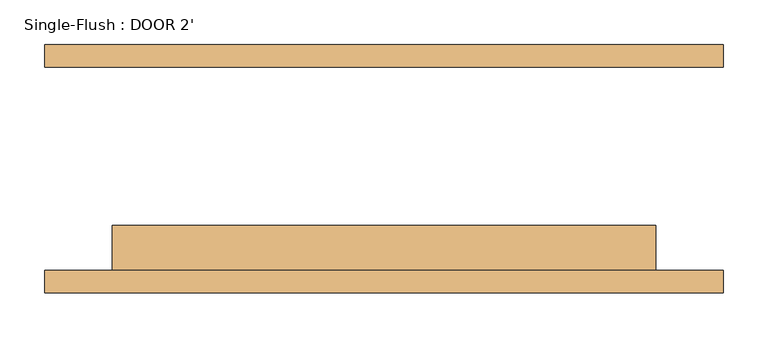
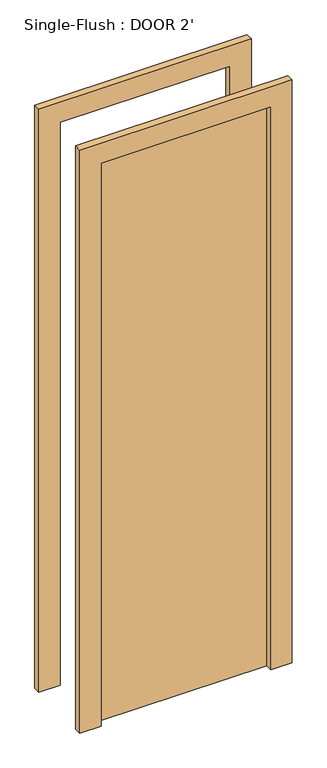
"""IFC4 building model written with IfcOpenShell, lengths in millimetres: door geometry, Single-Flush : DOOR 2'."""

from ifc_helpers import new_model, si_unit, frame, origin, origin_with_axes, place, context, project, spatial, polyline, outline, extrude, source, transform, mapped, element, save


def single_flush_door_2_4a3212df(model_context):
    return source(origin(), model_context, "Body", "SweptSolid", [
        extrude(outline(polyline([(2209.8, -381.0), (0.0, -381.0), (0.0, -304.8), (2133.6, -304.8), (2133.6, 304.8), (0.0, 304.8), (0.0, 381.0), (2209.8, 381.0), (2209.8, -381.0)])), frame((0.0, -139.7, 0.0), z_axis=(0.0, 1.0, 0.0), x_axis=(0.0, 0.0, 1.0)), (0.0, 0.0, 1.0), 25.4),
        extrude(outline(polyline([(2209.8, 381.0), (2209.8, -381.0), (0.0, -381.0), (0.0, -304.8), (2133.6, -304.8), (2133.6, 304.8), (0.0, 304.8), (0.0, 381.0), (2209.8, 381.0)])), frame((0.0, 114.3, 0.0), z_axis=(0.0, 1.0, 0.0), x_axis=(0.0, 0.0, 1.0)), (0.0, 0.0, 1.0), 25.4),
        extrude(outline(polyline([(304.8, -63.5), (304.8, -114.3), (-304.8, -114.3), (-304.8, -63.5), (304.8, -63.5)])), origin_with_axes(), (0.0, 0.0, 1.0), 2133.6),
    ])


if __name__ == "__main__":
    model = new_model("IFC4")
    model_context = context("Model", 3, world=origin())
    ifc_project = project(units=[si_unit("LENGTHUNIT", "METRE", prefix="MILLI")], contexts=[model_context])
    site = spatial("IfcSite", under=ifc_project)
    building = spatial("IfcBuilding", under=site)
    placement = place(None, origin())
    single_flush_door_2_shape = single_flush_door_2_4a3212df(model_context)
    element("IfcDoor", 1, ObjectType="Single-Flush : DOOR 2'", at=placement, inside=building, context=model_context, shape_type="MappedRepresentation", body=[
        mapped(single_flush_door_2_shape, transform((0.0, 0.0, 0.0), x_axis=(1.0, 0.0, 0.0), y_axis=(0.0, 1.0, 0.0), z_axis=(0.0, 0.0, 1.0))),
    ])
    save(model, "model.ifc")

# Revit data of these elements
# Type "Single-Flush : DOOR 2'"
#   Type Mark = "10"
#   Construction Type Id = "MDOOR"
#   Assembly Code = "C1020"
#   Analytic Construction = "Metal"
#   Thickness = 0' - 2"
#   Heat Transfer Coefficient (U) = 0.651978 BTU/(h·ft²·°F)
#   Height = 7' - 0"
#   Trim Projection Ext = 0' - 1"
#   Trim Projection Int = 0' - 1"
#   Trim Width = 0' - 3"
#   Width = 2' - 0"
#   Define Thermal Properties by = 1
#   Door Material = Door - Panel
#   Frame Material = Door - Frame
#   Visual Light Transmittance = 0
#   Solar Heat Gain Coefficient = 0
#   Function = (empty or 0)
#   Wall Closure = (empty or 0)
# Element 1 (IfcDoor, "Single-Flush : DOOR 2'")
#   Materials on its faces: "Door - Frame", "Door - Panel"
# Materials
#   "Door - Panel": class "Wood", colour RGB 210 159 95, transparency 0, Cost = 0
#   "Door - Frame": colour RGB 118 70 51, transparency 0, Cost = 0
